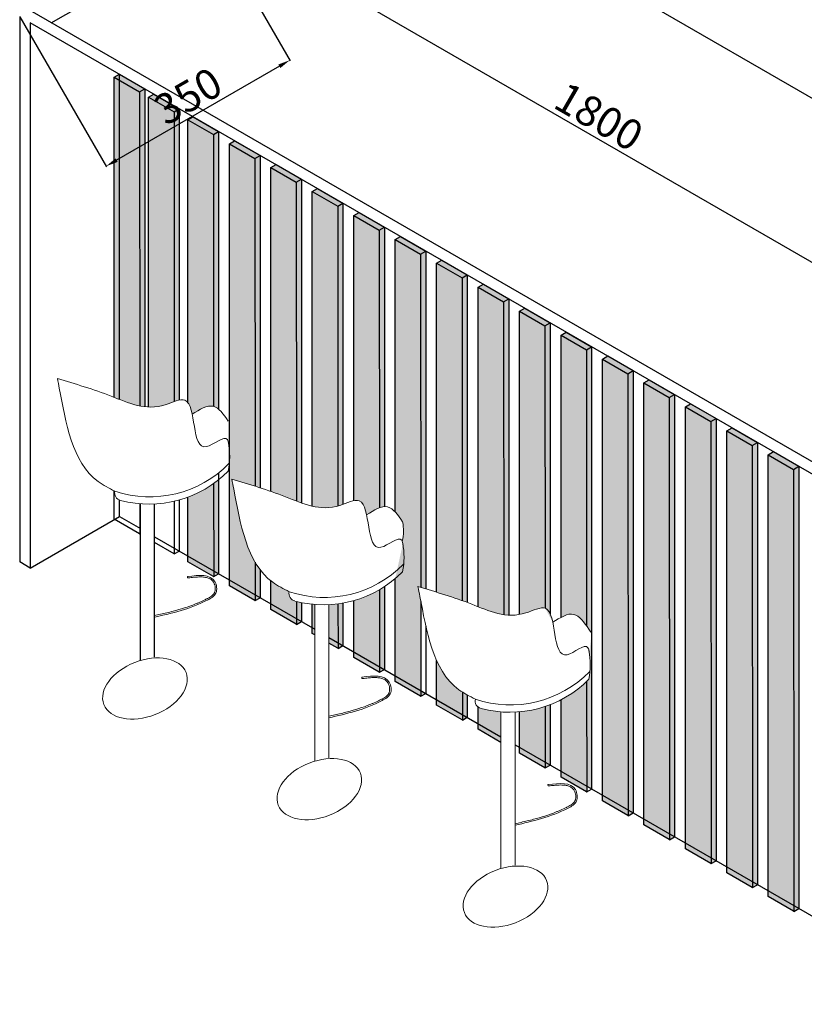
# Model space of a CAD drawing. Units: centimetres. Extents: x 209356 to 217348, y 253987 to 259034.
# Tile 1 of 7: x 209674 to 210968, y 254147 to 255772. Entities that reach past the tile are written whole.
import ezdxf

# ---------------------------------------------------------------- set-up
doc = ezdxf.new("R2010")
doc.units = ezdxf.units.CM
for name, color, linetype, lineweight in [('A-ANNO-DIMS', 2, 'Continuous', 18), ('A-ELEV', 7, 'Continuous', 25), ('A-ELEV-PATT', 32, 'Continuous', 13), ('A-FURN', 8, 'Continuous', 18)]:
    doc.layers.add(name, color=color, linetype=linetype, lineweight=lineweight)
doc.styles.get("Standard").update_dxf_attribs({"font": 'arial.ttf'})
doc.dimstyles.new('ISO-25', dxfattribs={"dimtxt": 50, "dimasz": 20, "dimexe": 1.25, "dimexo": 0.625, "dimtad": 1, "dimdec": 1, "dimtxsty": 'Standard', "dimcen": 2.5, "dimadec": 0, "dimazin": 0, "dimtfac": 1, "dimtdec": 1, "dimtmove": 0, "dimatfit": 3, "dimfxl": 1, "dimarcsym": 0})

# ---------------------------------------------------------------- blocks, each defined once
blk = doc.blocks.new('WOOD CHAIR')
for p, q in [((209213.3, 254105.5), (209213.3, 254643.6)), ((209261.5, 254116.4), (209261.5, 254642.8))]:
    blk.add_line(p, q)
for centre, radius, start, end in [((209261.7, 254806), 258.1, 348.8064, 10.7702), ((209245.8, 255048.2), 380.5, 251.5317, 315.539), ((209244, 255022.5), 380.1, 254.9145, 315.4643), ((209150.6, 254681), 26.1, 166.1036, 257.5958), ((209377.2, 254391.6), 2.77, 121.9926, 251.3474)]:
    blk.add_arc(centre, radius, start, end)
blk.add_ellipse((209228.8, 254009), major_axis=(141.2, 54.9), ratio=0.635047)
for points, knots in [([(209125.3, 254687.3), (209105.6, 254697.3), (208981, 254760.6), (208955.4, 254939), (208930.3, 255063), (208928.1, 255074)], [0, 0, 0, 0, 65.309963, 412.887053, 447.003391, 447.003391, 447.003391, 447.003391]), ([(208928.1, 255074), (208989.8, 255055.8), (209111.4, 255019.8), (209252.6, 254951.6), (209416.2, 255043.3), (209376.8, 254762.6), (209509.8, 254888.5), (209515.5, 254853.7), (209516.6, 254847.1)], [0, 0, 0, 0, 194.243648, 382.765289, 451.97711, 627.912461, 703.167603, 720.786202, 720.786202, 720.786202, 720.786202]), ([(209391.1, 254951.4), (209416.7, 254967.6), (209466.1, 254998.8), (209498.9, 254951.1), (209514.8, 254928)], [0, 0, 0, 0, 77.238961, 149.434731, 149.434731, 149.434731, 149.434731]), ([(209261.5, 254254.3), (209322.4, 254268), (209395, 254284.4), (209480, 254333), (209469.6, 254404.9), (209414.5, 254398.5), (209375.7, 254393.9)], [0, 0, 0, 0, 191.8386, 228.622109, 268.524723, 363.218072, 363.218072, 363.218072, 363.218072]), ([(209261.5, 254259.4), (209268.3, 254260.9), (209275.2, 254262.5), (209296.5, 254267.4), (209311, 254270.8), (209351.3, 254281.4), (209377.1, 254289.4), (209406.1, 254301.1), (209409.4, 254302.4), (209419.3, 254306.7), (209425.9, 254309.7), (209434.3, 254313.8), (209436.1, 254314.7), (209439.3, 254316.3), (209440.7, 254317), (209443.4, 254318.4), (209444.8, 254319.1), (209448.8, 254321.3), (209451.4, 254322.8), (209456.2, 254325.9), (209458.4, 254327.5), (209462.3, 254331), (209464, 254332.8), (209466.2, 254335.7), (209466.8, 254336.8), (209467.7, 254338.5), (209468, 254339.2), (209468.6, 254340.6), (209468.8, 254341.4), (209469.5, 254343.7), (209469.8, 254345.3), (209470.4, 254349.8), (209470.4, 254352.9), (209469.8, 254359), (209469.2, 254362), (209467.4, 254367.9), (209466.3, 254370.6), (209463.9, 254375), (209462.7, 254376.7), (209460.1, 254379.9), (209458.7, 254381.2), (209455.6, 254383.8), (209454, 254384.9), (209450.4, 254386.8), (209448.5, 254387.7), (209442.5, 254389.9), (209438.1, 254390.9), (209428.4, 254392.2), (209423.3, 254392.4), (209412.3, 254392.4), (209406.6, 254392), (209394.8, 254391.1), (209388.8, 254390.4), (209380.6, 254389.5), (209378.4, 254389.2), (209376.3, 254389)], [1.156813, 1.156813, 1.156813, 1.156813, 22.810617, 22.810617, 68.431852, 68.431852, 150.393922, 150.393922, 160.904538, 160.904538, 181.925769, 181.925769, 187.749873, 187.749873, 192.127257, 192.127257, 196.504641, 196.504641, 205.259408, 205.259408, 214.014175, 214.014175, 222.768943, 222.768943, 227.399514, 227.399514, 230.222361, 230.222361, 233.045208, 233.045208, 238.690903, 238.690903, 248.267073, 248.267073, 257.843243, 257.843243, 267.419412, 267.419412, 275.074878, 275.074878, 282.730344, 282.730344, 290.38581, 290.38581, 298.041276, 298.041276, 313.03296, 313.03296, 328.024645, 328.024645, 343.016329, 343.016329, 358.008014, 358.008014, 363.218072, 363.218072, 363.218072, 363.218072])]:
    blk.add_open_spline(points, degree=3, knots=knots)
blk = doc.blocks.new('FLUTED-PANEL')
for p, q in [((0, 753.9), (8.7, 758.9)), ((0, 24.5), (0, 753.9)), ((0, 753.9), (41.9, 729.7)), ((8.7, 758.9), (50.6, 734.7)), ((41.9, 729.7), (50.6, 734.7)), ((50.6, 734.7), (50.6, 4.7)), ((41.9, 729.7), (42.4, 0)), ((41.9, 0.3), (0, 24.5)), ((41.9, 0.3), (42.4, 0)), ((42.4, 0), (50.6, 4.7))]:
    blk.add_line(p, q)
blk = doc.blocks.new('*D12')
at = {"layer": 'A-ANNO-DIMS', "color": 0, "lineweight": -2, "transparency": 16777216}
for p, q in [((209691.8, 255787.1), (209834.6, 256034.4)), ((209851.3, 256023.4), (211375.5, 255143.4)), ((211250.7, 254887.1), (211393.5, 255134.4))]:
    blk.add_line(p, q, dxfattribs=at)
at = {"layer": 'A-ANNO-DIMS', "color": 0, "transparency": 16777216}
for points in [[(209853, 256026.3), (209849.6, 256020.5), (209834, 256033.4)], [(211377.2, 255146.3), (211373.9, 255140.5), (211392.8, 255133.4)]]:
    blk.add_solid(points, dxfattribs=at)
at = {"layer": 'Defpoints', "color": 0, "transparency": 16777216}
for p in [(209691.5, 255786.5), (211392.8, 255133.4), (211250.3, 254886.5)]:
    blk.add_point(p, dxfattribs=at)
at = {"layer": 'A-ANNO-DIMS', "color": 0, "transparency": 16777216, "insert": (210626.5, 255606), "char_height": 50, "attachment_point": 5, "rotation": 330}
blk.add_mtext('1800', dxfattribs=at)
blk = doc.blocks.new('*D34')
at = {"layer": 'A-ANNO-DIMS', "color": 0, "lineweight": -2, "transparency": 16777216}
for p, q in [((209977.6, 255951), (210120.4, 255703.6)), ((209674.5, 255776), (209817.3, 255528.6)), ((210102.5, 255694.7), (209834, 255539.7))]:
    blk.add_line(p, q, dxfattribs=at)
at = {"layer": 'A-ANNO-DIMS', "color": 0, "transparency": 16777216}
for points in [[(210100.8, 255697.6), (210104.1, 255691.8), (210119.8, 255704.7)], [(209832.3, 255542.6), (209835.7, 255536.8), (209816.7, 255529.7)]]:
    blk.add_solid(points, dxfattribs=at)
at = {"layer": 'Defpoints', "color": 0, "transparency": 16777216}
for p in [(209977.3, 255951.5), (209674.2, 255776.5), (209816.7, 255529.7)]:
    blk.add_point(p, dxfattribs=at)
at = {"layer": 'A-ANNO-DIMS', "color": 0, "transparency": 16777216, "insert": (209955.1, 255639.9), "char_height": 50, "attachment_point": 5, "rotation": 30}
blk.add_mtext('350', dxfattribs=at)

msp = doc.modelspace()

# ---------------------------------------------------------------- hatches: boundary and pattern name
at = {"layer": 'A-ELEV-PATT'}
h = msp.add_hatch(color=256, dxfattribs=at)
h.dxf.hatch_style = 1
h.paths.add_polyline_path([(209838.7169, 255681.5492), (209830.0636, 255676.5532), (209871.9793, 255652.3531), (209880.6326, 255657.3491)])
h.paths.add_polyline_path([(209872.3394, 255134.0549), (209880.6326, 255132.7439), (209880.6326, 255657.3491), (209871.9793, 255652.3531)])
h.paths.add_polyline_path([(209871.6996, 255134.2031), (209872.3394, 255134.0785), (209871.9793, 255652.3531), (209830.0636, 255676.5532), (209830.0636, 255148.2775), (209832.6333, 255147.2538), (209835.2039, 255146.2291), (209837.7762, 255145.2078), (209840.3508, 255144.1942), (209842.9285, 255143.1925), (209845.5101, 255142.2073), (209848.0963, 255141.2426), (209850.6877, 255140.3029), (209853.2852, 255139.3926), (209855.8896, 255138.5158), (209858.5014, 255137.677), (209861.1216, 255136.8804), (209863.7507, 255136.1304), (209866.3896, 255135.4313), (209869.039, 255134.7874)])
h = msp.add_hatch(color=256, dxfattribs=at)
h.dxf.hatch_style = 1
h.paths.add_polyline_path([(209895.4569, 255648.7903), (209886.8036, 255643.7943), (209928.7193, 255619.5942), (209937.3726, 255624.5902)])
h.paths.add_polyline_path([(209886.8036, 255132.2353), (209889.7902, 255132.1482), (209892.7967, 255132.1701), (209895.8239, 255132.3066), (209898.873, 255132.5631), (209901.9447, 255132.9452), (209905.0401, 255133.4584), (209908.16, 255134.1083), (209911.3054, 255134.9002), (209914.4774, 255135.8398), (209917.6725, 255136.9213), (209920.8723, 255138.0978), (209924.0546, 255139.3129), (209927.1973, 255140.5103), (209929.0517, 255141.1863), (209928.7193, 255619.5942), (209886.8036, 255643.7943)])
h = msp.add_hatch(color=256, dxfattribs=at)
h.dxf.hatch_style = 1
edge = h.paths.add_edge_path()
edge.add_line((209937.3726, 255624.5902), (209928.7193, 255619.5942))
edge.add_line((209928.7193, 255619.5942), (209929.0517, 255141.1956))
edge.add_spline(control_points=[(209929.0517, 255141.1956), (209931.9533, 255142.248), (209934.7548, 255143.1561), (209937.3726, 255143.7067)], knot_values=[411.187631291, 411.187631291, 411.187631291, 411.187631291, 428.578941434, 428.578941434, 428.578941434, 428.578941434], degree=3, periodic=0)
edge.add_line((209937.3726, 255143.7067), (209937.3726, 255624.5902))
edge = h.paths.add_edge_path()
edge.add_line((209993.6447, 255582.1096), (209951.7289, 255606.3096))
edge.add_line((209951.7289, 255606.3096), (209951.7289, 255139.4147))
edge.add_spline(control_points=[(209951.7289, 255139.4147), (209954.9954, 255135.0962), (209957.0859, 255128.2201), (209958.7321, 255120.3781)], knot_values=[468.970685224, 468.970685224, 468.970685224, 468.970685224, 508.024917649, 508.024917649, 508.024917649, 508.024917649], degree=3, periodic=0)
edge.add_spline(control_points=[(209958.7321, 255120.3781), (209971.0125, 255128.1269), (209983.5055, 255136.01), (209993.7821, 255133.4155), (209993.9564, 255133.3684)], knot_values=[0, 0, 0, 0, 77.238961281, 78.57658104, 78.57658104, 78.57658104, 78.57658104], degree=3, periodic=0)
edge.add_line((209993.9564, 255133.3684), (209993.6447, 255582.1096))
h = msp.add_hatch(color=256, dxfattribs=at)
h.dxf.hatch_style = 1
h.paths.add_polyline_path([(209960.3823, 255611.3056), (209951.7289, 255606.3096), (209993.6447, 255582.1096), (210002.298, 255587.1056)])
edge = h.paths.add_edge_path()
edge.add_arc((209888.0616, 255154.5395), 182.5816, 290.4081991, 305.4836992)
edge.add_line((209994.045, 255005.8668), (209994.1516, 254852.4022))
edge.add_line((209994.1516, 254852.4022), (209951.7289, 254876.895))
edge.add_line((209951.7289, 254876.895), (209951.7289, 254983.4181))
edge = h.paths.add_edge_path()
edge.add_arc((209888.0616, 255154.5395), 182.5816, 305.4836992, 308.7315997)
edge.add_line((210002.298, 255012.1102), (210002.298, 254857.1056))
edge.add_line((210002.298, 254857.1056), (209994.1516, 254852.4022))
edge.add_line((209994.1516, 254852.4022), (209994.045, 255005.8668))
h.paths.add_polyline_path([(209993.9565, 255133.3142), (209994.8652, 255133.094), (209997.4235, 255132.0135), (209999.8981, 255130.5369), (210002.298, 255128.7074), (210002.298, 255587.1056), (209993.6447, 255582.1096)])
h.paths.add_polyline_path([(210001.5192, 255076.2748), (210001.1006, 255076.0389), (210002.1063, 255076.5853)])
h.paths.add_polyline_path([(209996.6216, 255073.4867), (209994.8818, 255072.491), (209995.4223, 255072.7972)])
h.paths.add_polyline_path([(209994.0875, 255072.0409), (209993.9991, 255071.9919), (209993.9991, 255071.9908)])
h.paths.add_polyline_path([(209999.286, 255075.0167), (209999.2266, 255074.9826), (209999.4643, 255075.1166)])
h.paths.add_polyline_path([(209993.9991, 255071.9857), (209994.3441, 255072.1832), (209993.9991, 255071.9919)])
h = msp.add_hatch(color=256, dxfattribs=at)
h.dxf.hatch_style = 1
edge = h.paths.add_edge_path()
edge.add_line((210062.018, 255542.6342), (210020.1023, 255566.8343))
edge.add_line((210020.1023, 255566.8343), (210020.1023, 255061.2706))
edge.add_arc((209896.5952, 255050.551), 123.9714, -4.9604263, 4.9604263, ccw=False)
edge.add_line((210020.1023, 255039.8315), (210020.1023, 254846.8263))
edge.add_line((210020.1023, 254846.8263), (210062.5184, 254822.3373))
edge.add_line((210062.5184, 254822.3373), (210062.481, 254876.2165))
edge.add_spline(control_points=[(210062.481, 254876.2165), (210042.2873, 254910.7685), (210034.11, 254963.1736), (210025.0707, 255007.8633), (210023.9948, 255013.1827)], knot_values=[160.382869641, 160.382869641, 160.382869641, 160.382869641, 412.887053283, 447.00339111, 447.00339111, 447.00339111, 447.00339111], degree=3, periodic=0)
edge.add_spline(control_points=[(210023.9948, 255013.1827), (210036.8013, 255009.3967), (210049.6079, 255005.6107), (210062.3939, 255001.6068)], knot_values=[0, 0, 0, 0, 83.916340246, 83.916340246, 83.916340246, 83.916340246], degree=3, periodic=0)
edge.add_line((210062.3939, 255001.6068), (210062.018, 255542.6342))
edge = h.paths.add_edge_path()
edge.add_line((210070.6713, 255547.6302), (210062.018, 255542.6342))
edge.add_line((210062.018, 255542.6342), (210062.3939, 255001.6068))
edge.add_spline(control_points=[(210062.3939, 255001.6068), (210065.154, 255000.7425), (210067.9133, 254999.868), (210070.6713, 254998.9811)], knot_values=[83.916340246, 83.916340246, 83.916340246, 83.916340246, 102.031847918, 102.031847918, 102.031847918, 102.031847918], degree=3, periodic=0)
edge.add_line((210070.6713, 254998.9811), (210070.6713, 255547.6302))
h = msp.add_hatch(color=256, dxfattribs=at)
h.dxf.hatch_style = 1
h.paths.add_polyline_path([(210028.7556, 255571.8303), (210020.1023, 255566.8343), (210062.018, 255542.6342), (210070.6713, 255547.6302)])
h.paths.add_polyline_path([(210062.5184, 254822.3373), (210020.1023, 254846.8263), (210020.1023, 254837.4196), (210062.5249, 254812.9269)])
h.paths.add_polyline_path([(210070.6713, 254817.6302), (210062.5184, 254822.3373), (210062.5249, 254812.9269)])
h = msp.add_hatch(color=256, dxfattribs=at)
h.dxf.hatch_style = 1
h.paths.add_polyline_path([(210097.1289, 255532.3549), (210088.4756, 255527.3589), (210130.3913, 255503.1589), (210139.0446, 255508.1548)])
h = msp.add_hatch(color=256, dxfattribs=at)
h.dxf.hatch_style = 1
edge = h.paths.add_edge_path()
edge.add_line((210130.3913, 255503.1589), (210088.4756, 255527.3589))
edge.add_line((210088.4756, 255527.3589), (210088.4756, 254993.0564))
edge.add_spline(control_points=[(210088.4756, 254993.0564), (210096.5563, 254990.2663), (210110.6625, 254985.1298), (210124.7103, 254979.3735), (210130.7568, 254977.0458)], knot_values=[141.052694506, 141.052694506, 141.052694506, 141.052694506, 194.243647816, 234.067349628, 234.067349628, 234.067349628, 234.067349628], degree=3, periodic=0)
edge.add_line((210130.7568, 254977.0458), (210130.3913, 255503.1589))
edge = h.paths.add_edge_path()
edge.add_line((210198.7647, 255463.6835), (210156.8489, 255487.8836))
edge.add_line((210156.8489, 255487.8836), (210156.8489, 254968.6697))
edge.add_spline(control_points=[(210156.8489, 254968.6697), (210170.3528, 254965.5595), (210184.2937, 254964.768), (210199.1084, 254968.8528)], knot_values=[290.654547314, 290.654547314, 290.654547314, 290.654547314, 377.058614809, 377.058614809, 377.058614809, 377.058614809], degree=3, periodic=0)
edge.add_line((210199.1084, 254968.8528), (210198.7647, 255463.6835))
edge = h.paths.add_edge_path()
edge.add_line((210267.138, 255424.2081), (210225.2222, 255448.4082))
edge.add_line((210225.2222, 255448.4082), (210225.2222, 254977.6598))
edge.add_spline(control_points=[(210225.2222, 254977.6598), (210228.6719, 254978.3656), (210239.4144, 254978.6135), (210244.0368, 254965.5476), (210246.3993, 254954.2934)], knot_values=[428.983516451, 428.983516451, 428.983516451, 428.983516451, 451.977109906, 508.024917649, 508.024917649, 508.024917649, 508.024917649], degree=3, periodic=0)
edge.add_spline(control_points=[(210246.3993, 254954.2934), (210253.5599, 254958.8116), (210260.7204, 254963.3299), (210267.4564, 254965.8411)], knot_values=[0, 0, 0, 0, 45.037191144, 45.037191144, 45.037191144, 45.037191144], degree=3, periodic=0)
edge.add_line((210267.4564, 254965.8411), (210267.138, 255424.2081))
h = msp.add_hatch(color=256, dxfattribs=at)
h.dxf.hatch_style = 1
edge = h.paths.add_edge_path()
edge.add_line((210139.0446, 255508.1548), (210130.3913, 255503.1589))
edge.add_line((210130.3913, 255503.1589), (210130.7568, 254977.0458))
edge.add_spline(control_points=[(210130.7568, 254977.0458), (210133.5114, 254975.9853), (210136.2727, 254974.9532), (210139.0446, 254973.9732)], knot_values=[234.067349628, 234.067349628, 234.067349628, 234.067349628, 252.209805879, 252.209805879, 252.209805879, 252.209805879], degree=3, periodic=0)
edge.add_line((210139.0446, 254973.9732), (210139.0446, 255508.1548))
edge = h.paths.add_edge_path()
edge.add_line((210207.418, 255468.6795), (210198.7647, 255463.6835))
edge.add_line((210198.7647, 255463.6835), (210199.1084, 254968.8528))
edge.add_spline(control_points=[(210199.1084, 254968.8528), (210200.0869, 254969.1225), (210202.8425, 254969.939), (210205.6292, 254970.9288), (210207.418, 254971.5931)], knot_values=[377.058614809, 377.058614809, 377.058614809, 377.058614809, 382.765289469, 393.068098738, 393.068098738, 393.068098738, 393.068098738], degree=3, periodic=0)
edge.add_line((210207.418, 254971.5931), (210207.418, 255468.6795))
edge = h.paths.add_edge_path()
edge.add_line((210275.7913, 255429.2041), (210267.138, 255424.2081))
edge.add_line((210267.138, 255424.2081), (210267.4564, 254965.8411))
edge.add_spline(control_points=[(210267.4564, 254965.8411), (210270.3225, 254966.9096), (210273.1117, 254967.6148), (210275.7913, 254967.802)], knot_values=[45.037191144, 45.037191144, 45.037191144, 45.037191144, 64.199838197, 64.199838197, 64.199838197, 64.199838197], degree=3, periodic=0)
edge.add_line((210275.7913, 254967.802), (210275.7913, 255429.2041))
h = msp.add_hatch(color=256, dxfattribs=at)
h.dxf.hatch_style = 1
h.paths.add_polyline_path([(210165.5022, 255492.8796), (210156.8489, 255487.8836), (210198.7647, 255463.6835), (210207.418, 255468.6795)])
h = msp.add_hatch(color=256, dxfattribs=at)
h.dxf.hatch_style = 1
h.paths.add_polyline_path([(210233.8755, 255453.4042), (210225.2222, 255448.4082), (210267.138, 255424.2081), (210275.7913, 255429.2041)])
edge = h.paths.add_edge_path()
edge.add_arc((210175.7288, 254988.4547), 182.5816, 300.1924839, 303.2328114)
edge.add_line((210275.7913, 254835.7342), (210275.7913, 254699.2041))
edge.add_line((210275.7913, 254699.2041), (210267.6449, 254694.5008))
edge.add_line((210267.6449, 254694.5008), (210267.5503, 254830.642))
edge = h.paths.add_edge_path()
edge.add_arc((210175.7288, 254988.4547), 182.5816, 285.7282758, 300.1924839)
edge.add_line((210267.5503, 254830.642), (210267.6449, 254694.5008))
edge.add_line((210267.6449, 254694.5008), (210225.2222, 254718.9936))
edge.add_line((210225.2222, 254718.9936), (210225.2222, 254812.7093))
h = msp.add_hatch(color=256, dxfattribs=at)
h.dxf.hatch_style = 1
edge = h.paths.add_edge_path()
edge.add_line((210335.5113, 255384.7328), (210293.5956, 255408.9329))
edge.add_line((210293.5956, 255408.9329), (210293.5956, 254959.1517))
edge.add_spline(control_points=[(210293.5956, 254959.1517), (210297.8374, 254954.6317), (210301.8122, 254948.8491), (210305.787, 254943.0666)], knot_values=[111.704744255, 111.704744255, 111.704744255, 111.704744255, 149.434731389, 149.434731389, 149.434731389, 149.434731389], degree=3, periodic=0)
edge.add_arc((210232.7205, 254928.0817), 74.5872, -13.5167625, 11.5898438, ccw=False)
edge.add_spline(control_points=[(210305.2418, 254910.6484), (210305.8981, 254908.8541), (210306.2766, 254906.5205), (210306.6552, 254904.1869)], knot_values=[707.821270708, 707.821270708, 707.821270708, 707.821270708, 720.786201866, 720.786201866, 720.786201866, 720.786201866], degree=3, periodic=0)
edge.add_arc((210184.2624, 254884.4663), 123.9714, 9.9291308, 11.134566, ccw=False)
edge.add_spline(control_points=[(210306.6552, 254904.1869), (210306.2766, 254906.5205), (210305.8981, 254908.8541), (210305.2418, 254910.6484)], knot_values=[707.821270708, 707.821270708, 707.821270708, 707.821270708, 720.786201866, 720.786201866, 720.786201866, 720.786201866], degree=3, periodic=0)
edge.add_arc((210184.2624, 254884.4663), 123.9714, -11.1935567, 10.3654744, ccw=False)
edge.add_arc((210175.7288, 254988.4547), 182.5816, 310.2074031, 315.4643031, ccw=False)
edge.add_line((210293.5956, 254849.0148), (210293.5956, 254688.9248))
edge.add_line((210293.5956, 254688.9248), (210336.0117, 254664.4359))
edge.add_line((210336.0117, 254664.4359), (210335.9095, 254811.4969))
edge.add_spline(control_points=[(210335.9095, 254811.4969), (210335.3731, 254814.2946), (210333.7804, 254822.5539), (210332.1599, 254830.5652), (210331.084, 254835.8846)], knot_values=[395.621930027, 395.621930027, 395.621930027, 395.621930027, 412.887053283, 447.00339111, 447.00339111, 447.00339111, 447.00339111], degree=3, periodic=0)
edge.add_spline(control_points=[(210331.084, 254835.8846), (210332.6872, 254835.4107), (210334.2904, 254834.9367), (210335.8936, 254834.4624)], knot_values=[0, 0, 0, 0, 10.505199123, 10.505199123, 10.505199123, 10.505199123], degree=3, periodic=0)
edge.add_line((210335.8936, 254834.4624), (210335.5113, 255384.7328))
h = msp.add_hatch(color=256, dxfattribs=at)
h.dxf.hatch_style = 1
h.paths.add_polyline_path([(210302.2489, 255413.9288), (210293.5956, 255408.9329), (210335.5113, 255384.7328), (210344.1646, 255389.7288)])
h.paths.add_polyline_path([(210336.0117, 254664.4359), (210293.5956, 254688.9248), (210293.5956, 254679.5182), (210336.0182, 254655.0255)])
h.paths.add_polyline_path([(210344.1646, 254659.7288), (210336.0117, 254664.4359), (210336.0182, 254655.0255)])
h = msp.add_hatch(color=256, dxfattribs=at)
h.dxf.hatch_style = 1
edge = h.paths.add_edge_path()
edge.add_line((210344.1646, 255389.7288), (210335.5113, 255384.7328))
edge.add_line((210335.5113, 255384.7328), (210335.8936, 254834.4624))
edge.add_spline(control_points=[(210335.8936, 254834.4624), (210338.6508, 254833.6465), (210341.4079, 254832.8294), (210344.1646, 254832.0088)], knot_values=[10.505199123, 10.505199123, 10.505199123, 10.505199123, 28.572517978, 28.572517978, 28.572517978, 28.572517978], degree=3, periodic=0)
edge.add_line((210344.1646, 254832.0088), (210344.1646, 255389.7288))
h = msp.add_hatch(color=256, dxfattribs=at)
h.dxf.hatch_style = 1
h.paths.add_polyline_path([(210370.6222, 255374.4535), (210361.9689, 255369.4575), (210403.8846, 255345.2574), (210412.5379, 255350.2534)])
h.paths.add_polyline_path([(210412.5379, 254620.2534), (210404.385, 254624.9605), (210404.3915, 254615.5501)])
h.paths.add_polyline_path([(210404.385, 254624.9605), (210361.9689, 254649.4495), (210361.9689, 254640.0428), (210404.3915, 254615.5501)])
h = msp.add_hatch(color=256, dxfattribs=at)
h.dxf.hatch_style = 1
edge = h.paths.add_edge_path()
edge.add_line((210403.8846, 255345.2574), (210361.9689, 255369.4575))
edge.add_line((210361.9689, 255369.4575), (210361.9689, 254826.6377))
edge.add_spline(control_points=[(210361.9689, 254826.6377), (210376.0935, 254822.3021), (210390.198, 254817.7529), (210404.2546, 254812.6966)], knot_values=[67.482286261, 67.482286261, 67.482286261, 67.482286261, 160.131888062, 160.131888062, 160.131888062, 160.131888062], degree=3, periodic=0)
edge.add_line((210404.2546, 254812.6966), (210403.8846, 255345.2574))
h = msp.add_hatch(color=256, dxfattribs=at)
h.dxf.hatch_style = 1
edge = h.paths.add_edge_path()
edge.add_line((210412.5379, 255350.2534), (210403.8846, 255345.2574))
edge.add_line((210403.8846, 255345.2574), (210404.2546, 254812.6966))
edge.add_spline(control_points=[(210404.2546, 254812.6966), (210407.0176, 254811.7027), (210409.7788, 254810.6893), (210412.5379, 254809.654)], knot_values=[160.131888062, 160.131888062, 160.131888062, 160.131888062, 178.343545798, 178.343545798, 178.343545798, 178.343545798], degree=3, periodic=0)
edge.add_line((210412.5379, 254809.654), (210412.5379, 255350.2534))
h = msp.add_hatch(color=256, dxfattribs=at)
h.dxf.hatch_style = 1
h.paths.add_polyline_path([(210438.9955, 255334.9781), (210430.3422, 255329.9821), (210472.2579, 255305.7821), (210480.9113, 255310.7781)])
h = msp.add_hatch(color=256, dxfattribs=at)
h.dxf.hatch_style = 1
edge = h.paths.add_edge_path()
edge.add_line((210472.2579, 255305.7821), (210430.3422, 255329.9821))
edge.add_line((210430.3422, 255329.9821), (210430.3422, 254802.6944))
edge.add_spline(control_points=[(210430.3422, 254802.6944), (210444.1853, 254797.1865), (210458.104, 254791.8527), (210472.6164, 254789.7267)], knot_values=[217.563869727, 217.563869727, 217.563869727, 217.563869727, 309.028485894, 309.028485894, 309.028485894, 309.028485894], degree=3, periodic=0)
edge.add_line((210472.6164, 254789.7267), (210472.2579, 255305.7821))
h = msp.add_hatch(color=256, dxfattribs=at)
h.dxf.hatch_style = 1
edge = h.paths.add_edge_path()
edge.add_line((210480.9113, 255310.7781), (210472.2579, 255305.7821))
edge.add_line((210472.2579, 255305.7821), (210472.6164, 254789.7267))
edge.add_spline(control_points=[(210472.6164, 254789.7267), (210475.359, 254789.3249), (210478.1228, 254789.0377), (210480.9113, 254788.8855)], knot_values=[309.028485894, 309.028485894, 309.028485894, 309.028485894, 326.313488296, 326.313488296, 326.313488296, 326.313488296], degree=3, periodic=0)
edge.add_line((210480.9113, 254788.8855), (210480.9113, 255310.7781))
h = msp.add_hatch(color=256, dxfattribs=at)
h.dxf.hatch_style = 1
h.paths.add_polyline_path([(210507.3688, 255295.5028), (210498.7155, 255290.5068), (210540.6313, 255266.3067), (210549.2846, 255271.3027)])
edge = h.paths.add_edge_path()
edge.add_arc((210482.818, 254811.1567), 182.5816, 274.9951075, 288.6044838)
edge.add_line((210541.0677, 254638.1162), (210541.1382, 254536.5994))
edge.add_line((210541.1382, 254536.5994), (210498.7155, 254561.0921))
edge.add_line((210498.7155, 254561.0921), (210498.7155, 254629.2685))
edge = h.paths.add_edge_path()
edge.add_arc((210482.818, 254811.1567), 182.5816, 288.6044838, 291.3483603)
edge.add_line((210549.2846, 254641.1031), (210549.2846, 254541.3027))
edge.add_line((210549.2846, 254541.3027), (210541.1382, 254536.5994))
edge.add_line((210541.1382, 254536.5994), (210541.0677, 254638.1162))
h = msp.add_hatch(color=256, dxfattribs=at)
h.dxf.hatch_style = 1
edge = h.paths.add_edge_path()
edge.add_line((210540.6313, 255266.3067), (210498.7155, 255290.5068))
edge.add_line((210498.7155, 255290.5068), (210498.7155, 254789.8817))
edge.add_spline(control_points=[(210498.7155, 254789.8817), (210502.1454, 254790.472), (210517.4101, 254794.1527), (210543.8007, 254808.9556), (210551.126, 254788.2496), (210553.4885, 254776.9953)], knot_values=[362.369570317, 362.369570317, 362.369570317, 362.369570317, 382.765289469, 451.977109906, 508.024917649, 508.024917649, 508.024917649, 508.024917649], degree=3, periodic=0)
edge.add_line((210540.955, 254800.2404), (210540.6313, 255266.3067))
edge = h.paths.add_edge_path(flags=17)
edge.add_line((210549.2846, 255271.3027), (210540.6313, 255266.3067))
edge.add_line((210540.6313, 255266.3067), (210540.955, 254800.2846))
edge.add_spline(control_points=[(210540.955, 254800.2846), (210541.1368, 254800.2232), (210544.7056, 254798.9022), (210547.3296, 254795.5258), (210549.2846, 254791.151)], knot_values=[450.415519807, 450.415519807, 450.415519807, 450.415519807, 451.977109906, 481.471652475, 481.471652475, 481.471652475, 481.471652475], degree=3, periodic=0)
edge.add_line((210549.2846, 254791.151), (210549.2846, 255271.3027))
h = msp.add_hatch(color=256, dxfattribs=at)
h.dxf.hatch_style = 1
h.paths.add_polyline_path([(210575.7422, 255256.0274), (210567.0888, 255251.0314), (210609.0046, 255226.8314), (210617.6579, 255231.8274)])
h.paths.add_polyline_path([(210609.505, 254506.5344), (210567.0888, 254531.0234), (210567.0888, 254521.6168), (210609.5115, 254497.124)])
h = msp.add_hatch(color=256, dxfattribs=at)
h.dxf.hatch_style = 1
edge = h.paths.add_edge_path()
edge.add_line((210609.0046, 255226.8314), (210567.0888, 255251.0314))
edge.add_line((210567.0888, 255251.0314), (210567.0888, 254785.1249))
edge.add_spline(control_points=[(210567.0888, 254785.1249), (210574.6127, 254789.1096), (210590.8871, 254794.7518), (210602.86, 254780.0604), (210609.3213, 254770.8967)], knot_values=[28.745104313, 28.745104313, 28.745104313, 28.745104313, 77.238961281, 138.209017936, 138.209017936, 138.209017936, 138.209017936], degree=3, periodic=0)
edge.add_line((210609.3213, 254770.8967), (210609.0046, 255226.8314))
edge = h.paths.add_edge_path()
edge.add_line((210617.6579, 255231.8274), (210609.0046, 255226.8314))
edge.add_line((210609.0046, 255226.8314), (210609.3213, 254770.8967))
edge.add_spline(control_points=[(210609.3213, 254770.8967), (210610.511, 254769.2095), (210611.6936, 254767.489), (210612.8762, 254765.7686)], knot_values=[138.209017936, 138.209017936, 138.209017936, 138.209017936, 149.434731389, 149.434731389, 149.434731389, 149.434731389], degree=3, periodic=0)
edge.add_arc((210567.5561, 254726.927), 59.6873, 32.9227648, 40.5982268, ccw=False)
edge.add_line((210617.6579, 254759.3675), (210617.6579, 255231.8274))
h = msp.add_hatch(color=256, dxfattribs=at)
h.dxf.hatch_style = 1
h.paths.add_polyline_path([(210644.1155, 255216.5521), (210635.4622, 255211.5561), (210677.3779, 255187.356), (210686.0312, 255192.352)])
h.paths.add_polyline_path([(210677.8848, 254457.6487), (210686.0312, 254462.352), (210686.0312, 255192.352), (210677.3779, 255187.356)])
h.paths.add_polyline_path([(210635.4622, 254482.1414), (210677.8848, 254457.6487), (210677.3779, 255187.356), (210635.4622, 255211.5561)])
h = msp.add_hatch(color=256, dxfattribs=at)
h.dxf.hatch_style = 1
h.paths.add_polyline_path([(210712.4888, 255177.0767), (210703.8355, 255172.0807), (210745.7512, 255147.8807), (210754.4045, 255152.8766)])
h.paths.add_polyline_path([(210746.2582, 254418.1733), (210754.4045, 254422.8766), (210754.4045, 255152.8766), (210745.7512, 255147.8807)])
h.paths.add_polyline_path([(210703.8355, 254442.6661), (210746.2582, 254418.1733), (210745.7512, 255147.8807), (210703.8355, 255172.0807)])
h = msp.add_hatch(color=256, dxfattribs=at)
h.dxf.hatch_style = 1
h.paths.add_polyline_path([(210780.8621, 255137.6014), (210772.2088, 255132.6054), (210814.1246, 255108.4053), (210822.7779, 255113.4013)])
h.paths.add_polyline_path([(210814.6315, 254378.698), (210822.7779, 254383.4013), (210822.7779, 255113.4013), (210814.1246, 255108.4053)])
h.paths.add_polyline_path([(210772.2088, 254403.1907), (210814.6315, 254378.698), (210814.1246, 255108.4053), (210772.2088, 255132.6054)])
h = msp.add_hatch(color=256, dxfattribs=at)
h.dxf.hatch_style = 1
h.paths.add_polyline_path([(210849.2354, 255098.126), (210840.5821, 255093.13), (210882.4979, 255068.9299), (210891.1512, 255073.9259)])
h.paths.add_polyline_path([(210883.0048, 254339.2226), (210891.1512, 254343.9259), (210891.1512, 255073.9259), (210882.4979, 255068.9299)])
h.paths.add_polyline_path([(210840.5821, 254363.7154), (210883.0048, 254339.2226), (210882.4979, 255068.9299), (210840.5821, 255093.13)])
h = msp.add_hatch(color=256, dxfattribs=at)
h.dxf.hatch_style = 1
h.paths.add_polyline_path([(210917.6088, 255058.6506), (210908.9555, 255053.6546), (210950.8712, 255029.4546), (210959.5245, 255034.4506)])
h.paths.add_polyline_path([(210951.3781, 254299.7473), (210959.5245, 254304.4506), (210959.5245, 255034.4506), (210950.8712, 255029.4546)])
h.paths.add_polyline_path([(210908.9555, 254324.24), (210951.3781, 254299.7473), (210950.8712, 255029.4546), (210908.9555, 255053.6546)])
h = msp.add_hatch(color=256, dxfattribs=at)
h.dxf.hatch_style = 1
edge = h.paths.add_edge_path()
edge.add_spline(control_points=[(210070.6713, 254863.862), (210067.7214, 254867.7766), (210065.0001, 254871.9062), (210062.481, 254876.2165)], knot_values=[128.883300955, 128.883300955, 128.883300955, 128.883300955, 160.382869641, 160.382869641, 160.382869641, 160.382869641], degree=3, periodic=0)
edge.add_line((210062.481, 254876.2165), (210062.5184, 254822.3373))
edge.add_line((210062.5184, 254822.3373), (210070.6713, 254817.6302))
edge.add_line((210070.6713, 254817.6302), (210070.6713, 254863.862))
h.paths.add_polyline_path([(210088.4756, 254807.3509), (210088.4756, 254797.9443), (210130.3913, 254773.7442), (210130.8983, 254773.4515), (210130.8917, 254782.8619)])
edge = h.paths.add_edge_path()
edge.add_arc((210175.7288, 254988.4547), 182.5816, 254.9144881, 255.7778696, ccw=False)
edge.add_arc((210130.9033, 254824.4104), 12.5379, 166.1035689, 257.5957769, ccw=False)
edge.add_spline(control_points=[(210118.7324, 254827.4216), (210109.2654, 254832.2301), (210098.6031, 254837.6458), (210089.4795, 254844.6095), (210088.4756, 254845.4091)], knot_values=[0, 0, 0, 0, 65.309963166, 73.556041403, 73.556041403, 73.556041403, 73.556041403], degree=3, periodic=0)
edge.add_line((210088.4756, 254845.4091), (210088.4756, 254807.3509))
edge.add_line((210088.4756, 254807.3509), (210130.8917, 254782.8619))
edge.add_line((210130.8917, 254782.8619), (210130.8718, 254811.4691))
h.paths.add_polyline_path([(210139.0446, 254809.5964, -0.011482161), (210130.8718, 254811.4691), (210130.8917, 254782.8619), (210139.0446, 254778.1548)])
h.paths.add_polyline_path([(210130.8917, 254782.8619), (210130.8983, 254773.4515), (210139.0446, 254778.1548)])
h = msp.add_hatch(color=256, dxfattribs=at)
h.dxf.hatch_style = 1
h.paths.add_polyline_path([(210161.0165, 254806.4668, -0.005730997), (210156.8489, 254806.8519), (210156.8489, 254767.8755), (210161.0165, 254765.4694)])
h.paths.add_polyline_path([(210161.0165, 254765.4694), (210156.8489, 254767.8755), (210156.8489, 254758.4689), (210161.0165, 254756.0627)])
h.paths.add_polyline_path([(210199.2206, 254807.3907, -0.020749851), (210184.1309, 254806.0665), (210184.1309, 254752.1243), (210199.265, 254743.3866)])
h.paths.add_polyline_path([(210184.1309, 254752.1243), (210184.1309, 254742.7176), (210198.7647, 254734.2688), (210199.2716, 254733.9762), (210199.265, 254743.3866)])
h.paths.add_polyline_path([(210207.418, 254808.6441, -0.011356196), (210199.2206, 254807.3907), (210199.265, 254743.3866), (210207.418, 254738.6795)])
h.paths.add_polyline_path([(210199.265, 254743.3866), (210199.2716, 254733.9762), (210207.418, 254738.6795)])
h = msp.add_hatch(color=256, dxfattribs=at)
h.dxf.hatch_style = 1
h.paths.add_polyline_path([(210617.6579, 254759.3675), (210613.7444, 254726.8889, -0.089013219), (210612.9647, 254683.1024, -0.006893451), (210609.3848, 254679.563), (210609.505, 254506.5344), (210617.6579, 254501.8274)])
h = msp.add_hatch(color=256, dxfattribs=at)
h.dxf.hatch_style = 1
edge = h.paths.add_edge_path()
edge.add_spline(control_points=[(210404.3594, 254661.8817), (210402.3989, 254663.1254), (210383.5593, 254675.8421), (210370.6424, 254694.5177), (210361.9689, 254713.7236)], knot_values=[50.655423077, 50.655423077, 50.655423077, 50.655423077, 65.309963166, 194.96587381, 194.96587381, 194.96587381, 194.96587381], degree=3, periodic=0)
edge.add_line((210361.9689, 254713.7236), (210361.9689, 254649.4495))
edge.add_line((210361.9689, 254649.4495), (210404.385, 254624.9605))
edge.add_line((210404.385, 254624.9605), (210404.3594, 254661.8817))
edge = h.paths.add_edge_path()
edge.add_spline(control_points=[(210412.5379, 254657.0641), (210409.7477, 254658.6055), (210407.0102, 254660.2001), (210404.3594, 254661.8817)], knot_values=[30.84038343, 30.84038343, 30.84038343, 30.84038343, 50.655423077, 50.655423077, 50.655423077, 50.655423077], degree=3, periodic=0)
edge.add_line((210404.3594, 254661.8817), (210404.385, 254624.9605))
edge.add_line((210404.385, 254624.9605), (210412.5379, 254620.2534))
edge.add_line((210412.5379, 254620.2534), (210412.5379, 254657.0641))
h = msp.add_hatch(color=256, dxfattribs=at)
h.dxf.hatch_style = 1
h.paths.add_polyline_path([(210609.3848, 254679.563, -0.071668587), (210567.0888, 254649.1861), (210567.0888, 254531.0234), (210609.505, 254506.5344)])
h = msp.add_hatch(color=256, dxfattribs=at)
h.dxf.hatch_style = 1
h.paths.add_polyline_path([(210468.1057, 254629.1688, -0.045688015), (210435.2993, 254634.8671, -0.110391257), (210430.3422, 254637.179), (210430.3422, 254609.9741), (210468.1057, 254588.1713)])
h.paths.add_polyline_path([(210430.3422, 254609.9741), (210430.3422, 254600.5675), (210468.1057, 254578.7647), (210468.1057, 254588.1713)])

# ---------------------------------------------------------------- linework, layer by layer
at = {"layer": 'A-ELEV'}
for p, q in [((211769.9535, 255186.5492), (210211.1078, 256086.5492)), ((209726.1336, 255766.5492), (210245.7488, 256066.5492)), ((209674.1721, 255776.5492), (209674.1721, 254876.5492)), ((211250.3383, 254886.5492), (209691.4926, 255786.5492)), ((211233.0178, 254876.5492), (209691.4926, 255766.5492)), ((209691.4926, 255766.5492), (209691.4926, 254866.5492)), ((209830.0636, 255676.5532), (209838.7169, 255681.5492)), ((209838.7169, 255681.5492), (209880.6326, 255657.3491)), ((209838.7169, 255144.8362), (209838.7169, 255681.5492)), ((209830.0636, 255676.5532), (209871.9793, 255652.3531)), ((209830.0636, 255148.2775), (209830.0636, 255676.5532)), ((209871.9793, 255652.3531), (209880.6326, 255657.3491)), ((209871.9793, 255652.3531), (209872.3394, 255134.0723)), ((209880.6326, 255657.3491), (209880.6326, 255132.7439)), ((209886.8036, 255643.7943), (209895.4569, 255648.7903)), ((209895.4569, 255648.7903), (209937.3726, 255624.5902)), ((209886.8036, 255643.7943), (209928.7193, 255619.5942)), ((209886.8036, 255132.2353), (209886.8036, 255643.7943)), ((209928.7193, 255619.5942), (209937.3726, 255624.5902)), ((209928.7193, 255619.5942), (209929.0517, 255141.1956)), ((209937.3726, 255624.5902), (209937.3726, 255143.7067)), ((209951.7289, 255606.3096), (209960.3823, 255611.3056)), ((209951.7289, 255606.3096), (209993.6447, 255582.1096)), ((209951.7289, 255139.4147), (209951.7289, 255606.3096)), ((209960.3823, 255611.3056), (210002.298, 255587.1056)), ((209993.6447, 255582.1096), (210002.298, 255587.1056)), ((209993.6447, 255582.1096), (209993.9564, 255133.3684)), ((210002.298, 255587.1056), (210002.298, 255128.7074)), ((210020.1023, 255566.8343), (210028.7556, 255571.8303)), ((210020.1023, 254837.4196), (210020.1023, 255566.8343)), ((210020.1023, 255566.8343), (210062.018, 255542.6342)), ((210028.7556, 255571.8303), (210070.6713, 255547.6302)), ((210062.018, 255542.6342), (210070.6713, 255547.6302)), ((210070.6713, 255547.6302), (210070.6713, 254998.9811)), ((210062.018, 255542.6342), (210062.3939, 255001.6068)), ((210088.4756, 255527.3589), (210097.1289, 255532.3549)), ((210097.1289, 255532.3549), (210139.0446, 255508.1548)), ((210088.4756, 255527.3589), (210130.3913, 255503.1589)), ((210088.4756, 254993.0564), (210088.4756, 255527.3589)), ((210130.3913, 255503.1589), (210139.0446, 255508.1548)), ((210130.3913, 255503.1589), (210130.7568, 254977.0458)), ((210139.0446, 255508.1548), (210139.0446, 254973.9732)), ((210156.8489, 255487.8836), (210165.5022, 255492.8796)), ((210156.8489, 255487.8836), (210198.7647, 255463.6835)), ((210156.8489, 254968.6697), (210156.8489, 255487.8836)), ((210165.5022, 255492.8796), (210207.418, 255468.6795)), ((210198.7647, 255463.6835), (210207.418, 255468.6795)), ((210207.418, 255468.6795), (210207.418, 254971.5931)), ((210198.7647, 255463.6835), (210199.1084, 254968.8528)), ((210225.2222, 255448.4082), (210233.8755, 255453.4042)), ((210233.8755, 255453.4042), (210275.7913, 255429.2041)), ((210225.2222, 255448.4082), (210267.138, 255424.2081)), ((210225.2222, 254977.6598), (210225.2222, 255448.4082)), ((210267.138, 255424.2081), (210275.7913, 255429.2041)), ((210267.138, 255424.2081), (210267.4564, 254965.8411)), ((210275.7913, 255429.2041), (210275.7913, 254967.802)), ((210293.5956, 255408.9329), (210302.2489, 255413.9288)), ((210293.5956, 255408.9329), (210335.5113, 255384.7328)), ((210293.5956, 254959.1517), (210293.5956, 255408.9329)), ((210302.2489, 255413.9288), (210344.1646, 255389.7288)), ((210335.5113, 255384.7328), (210344.1646, 255389.7288)), ((210344.1646, 255389.7288), (210344.1646, 254832.0088)), ((210335.5113, 255384.7328), (210335.8936, 254834.4624)), ((210361.9689, 255369.4575), (210370.6222, 255374.4535)), ((210361.9689, 255369.4575), (210403.8846, 255345.2574)), ((210361.9689, 254826.6377), (210361.9689, 255369.4575)), ((210370.6222, 255374.4535), (210412.5379, 255350.2534)), ((210403.8846, 255345.2574), (210412.5379, 255350.2534)), ((210403.8846, 255345.2574), (210404.2546, 254812.6966)), ((210412.5379, 255350.2534), (210412.5379, 254809.654)), ((210430.3422, 255329.9821), (210438.9955, 255334.9781)), ((210430.3422, 255329.9821), (210472.2579, 255305.7821)), ((210430.3422, 254802.6944), (210430.3422, 255329.9821)), ((210438.9955, 255334.9781), (210480.9113, 255310.7781)), ((210472.2579, 255305.7821), (210480.9113, 255310.7781)), ((210472.2579, 255305.7821), (210472.6164, 254789.7267)), ((210480.9113, 255310.7781), (210480.9113, 254788.8855)), ((210498.7155, 255290.5068), (210507.3688, 255295.5028)), ((210498.7155, 255290.5068), (210540.6313, 255266.3067)), ((210498.7155, 254789.8817), (210498.7155, 255290.5068)), ((210507.3688, 255295.5028), (210549.2846, 255271.3027)), ((210540.6313, 255266.3067), (210549.2846, 255271.3027)), ((210549.2846, 255271.3027), (210549.2846, 254791.151)), ((210540.6313, 255266.3067), (210540.955, 254800.2846)), ((210567.0888, 255251.0314), (210575.7422, 255256.0274)), ((210575.7422, 255256.0274), (210617.6579, 255231.8274)), ((210567.0888, 255251.0314), (210609.0046, 255226.8314)), ((210567.0888, 254785.1249), (210567.0888, 255251.0314)), ((210609.0046, 255226.8314), (210617.6579, 255231.8274)), ((210609.0046, 255226.8314), (210609.3213, 254770.8967)), ((210617.6579, 255231.8274), (210617.6579, 254501.8274)), ((210002.298, 255023.4857), (210002.298, 254857.1056)), ((209994.045, 255005.8668), (209994.1516, 254852.4022)), ((209830.0636, 254947.1385), (209830.0636, 254994.0151)), ((209838.7169, 254951.5492), (209838.7169, 254978.8)), ((209951.7289, 254876.895), (209951.7289, 254983.4181)), ((209872.4515, 254972.6264), (209872.4862, 254922.6458)), ((209873.3493, 254714.0678), (209873.3493, 254972.5516)), ((209896.4637, 254719.3303), (209896.4637, 254972.1513)), ((209929.166, 254976.6449), (209929.2262, 254889.8869)), ((209937.3726, 254978.7428), (209937.3726, 254894.5902)), ((209691.4926, 254866.5492), (209838.7169, 254951.5492)), ((209871.9793, 254922.9384), (209830.0636, 254947.1385)), ((209838.7169, 254951.5492), (209873.3493, 254931.5541)), ((209871.9793, 254922.9384), (209872.4862, 254922.6458)), ((209872.4862, 254922.6458), (209873.3493, 254923.1441)), ((209896.4637, 254918.209), (210161.0165, 254765.4694)), ((209928.7193, 254890.1796), (209896.4637, 254908.8024)), ((209928.7193, 254890.1796), (209929.2262, 254889.8869)), ((209929.2262, 254889.8869), (209937.3726, 254894.5902)), ((209691.4926, 254866.5492), (209674.1721, 254876.5492)), ((209993.6447, 254852.6949), (209951.7289, 254876.895)), ((210062.481, 254876.2165), (210062.5249, 254812.9269)), ((209993.6447, 254852.6949), (209994.1516, 254852.4022)), ((209994.1516, 254852.4022), (210002.298, 254857.1056)), ((210070.6713, 254863.862), (210070.6713, 254817.6302)), ((210293.5956, 254679.5182), (210293.5956, 254849.0148)), ((210062.018, 254813.2196), (210020.1023, 254837.4196)), ((210088.4756, 254797.9443), (210088.4756, 254845.4091)), ((210275.7913, 254835.7342), (210275.7913, 254699.2041)), ((210062.5249, 254812.9269), (210070.6713, 254817.6302)), ((210267.5503, 254830.642), (210267.6449, 254694.5008)), ((210062.018, 254813.2196), (210062.5249, 254812.9269)), ((210130.8718, 254811.4691), (210130.8983, 254773.4515)), ((210139.0446, 254809.5964), (210139.0446, 254778.1548)), ((210156.8489, 254758.4689), (210156.8489, 254806.8519)), ((210199.2206, 254807.3907), (210199.2716, 254733.9762)), ((210207.418, 254808.6441), (210207.418, 254738.6795)), ((210225.2222, 254718.9936), (210225.2222, 254812.7093)), ((210335.9095, 254811.4969), (210336.0182, 254655.0255)), ((210130.3913, 254773.7442), (210088.4756, 254797.9443)), ((210130.3913, 254773.7442), (210130.8983, 254773.4515)), ((210130.8983, 254773.4515), (210139.0446, 254778.1548)), ((210344.1646, 254770.4559), (210344.1646, 254659.7288)), ((210161.0165, 254756.0627), (210156.8489, 254758.4689)), ((210184.1309, 254752.1243), (210468.1057, 254588.1713)), ((210198.7647, 254734.2688), (210184.1309, 254742.7176)), ((210199.2716, 254733.9762), (210207.418, 254738.6795)), ((210198.7647, 254734.2688), (210199.2716, 254733.9762)), ((210267.138, 254694.7935), (210225.2222, 254718.9936)), ((210361.9689, 254640.0428), (210361.9689, 254713.7236)), ((210267.138, 254694.7935), (210267.6449, 254694.5008)), ((210267.6449, 254694.5008), (210275.7913, 254699.2041)), ((210335.5113, 254655.3181), (210293.5956, 254679.5182)), ((210609.3848, 254679.563), (210609.5115, 254497.124)), ((210335.5113, 254655.3181), (210336.0182, 254655.0255)), ((210336.0182, 254655.0255), (210344.1646, 254659.7288)), ((210404.3594, 254661.8817), (210404.3915, 254615.5501)), ((210412.5379, 254657.0641), (210412.5379, 254620.2534)), ((210403.8846, 254615.8428), (210361.9689, 254640.0428)), ((210541.0677, 254638.1162), (210541.1382, 254536.5994)), ((210549.2846, 254641.1031), (210549.2846, 254541.3027)), ((210567.0888, 254521.6168), (210567.0888, 254649.1861)), ((210430.3422, 254600.5675), (210430.3422, 254637.179)), ((210498.7155, 254561.0921), (210498.7155, 254629.2685)), ((210403.8846, 254615.8428), (210404.3915, 254615.5501)), ((210404.3915, 254615.5501), (210412.5379, 254620.2534)), ((210468.1057, 254578.7647), (210430.3422, 254600.5675)), ((210491.2201, 254574.8262), (211233.0178, 254146.5492)), ((210540.6313, 254536.8921), (210498.7155, 254561.0921)), ((210541.1382, 254536.5994), (210549.2846, 254541.3027)), ((210540.6313, 254536.8921), (210541.1382, 254536.5994)), ((210609.0046, 254497.4167), (210567.0888, 254521.6168)), ((210609.0046, 254497.4167), (210609.5115, 254497.124)), ((210609.5115, 254497.124), (210617.6579, 254501.8274))]:
    msp.add_line(p, q, dxfattribs=at)
at = {"layer": 'A-FURN'}
for centre, radius, start, end in [((209896.5952, 255050.551), 123.9714, 348.8064433, 10.7701696), ((209888.9575, 255166.8472), 182.7528, 251.5317225, 315.5389761), ((209888.0616, 255154.5395), 182.5816, 254.9144881, 315.4643031), ((209843.2361, 254990.4951), 12.5379, 166.1035689, 257.5957769), ((210232.7205, 254928.0817), 74.5872, 346.4832375, 11.5898438), ((209952.0505, 254851.4908), 1.3284, 121.9925562, 251.3473535), ((210567.5561, 254726.927), 59.6873, 32.9227648, 40.5982268)]:
    msp.add_arc(centre, radius, start, end, dxfattribs=at)
msp.add_ellipse((209880.7961, 254667.7346), major_axis=(67.8132, 26.3545), ratio=0.635046934, dxfattribs=at)
for points, knots in [([(209831.0651, 254993.5063), (209821.5982, 254998.3149), (209761.7483, 255028.7142), (209749.4411, 255114.4346), (209737.4035, 255173.948), (209736.3276, 255179.2674)], [0, 0, 0, 0, 31.368446316, 198.310100598, 214.696214749, 214.696214749, 214.696214749, 214.696214749]), ([(209736.3276, 255179.2674), (209765.9713, 255170.5039), (209824.3854, 255153.2352), (209892.1917, 255120.4488), (209970.7662, 255164.5226), (209951.8747, 255029.6999), (210015.7615, 255090.1595), (210018.4735, 255073.4429), (210018.988, 255070.2717)], [0, 0, 0, 0, 93.295435235, 183.842584689, 217.085097294, 301.587037687, 337.732164143, 346.194396421, 346.194396421, 346.194396421, 346.194396421]), ([(209958.7321, 255120.3781), (209971.0125, 255128.1269), (209994.7714, 255143.1187), (210010.5141, 255120.2161), (210018.1198, 255109.1513)], [0, 0, 0, 0, 37.09795708, 71.773663957, 71.773663957, 71.773663957, 71.773663957]), ([(209896.4637, 254785.5337), (209925.7237, 254792.1453), (209960.594, 254800.0247), (210001.4117, 254823.348), (209996.4297, 254857.8895), (209969.9654, 254854.7947), (209951.3467, 254852.6174)], [0, 0, 0, 0, 92.140288038, 109.80744756, 128.972716333, 174.454034754, 174.454034754, 174.454034754, 174.454034754]), ([(209896.4637, 254787.9958), (209899.7661, 254788.742), (209903.0658, 254789.4883), (209913.3086, 254791.8446), (209920.2419, 254793.4964), (209939.595, 254798.5811), (209951.985, 254802.3845), (209965.9248, 254808.0136), (209967.5087, 254808.673), (209972.2588, 254810.7136), (209975.4235, 254812.1575), (209979.4627, 254814.1223), (209980.3389, 254814.5558), (209981.8733, 254815.3283), (209982.5323, 254815.6643), (209983.8476, 254816.3437), (209984.5001, 254816.6856), (209986.4263, 254817.7251), (209987.6682, 254818.4371), (209989.9803, 254819.9312), (209991.0497, 254820.7132), (209992.9369, 254822.3664), (209993.7537, 254823.2363), (209994.7746, 254824.651), (209995.0865, 254825.156), (209995.5201, 254826.0024), (209995.6681, 254826.3303), (209995.9377, 254827.0152), (209996.0587, 254827.3704), (209996.3796, 254828.4699), (209996.5372, 254829.2482), (209996.809, 254831.4291), (209996.816, 254832.889), (209996.5257, 254835.8225), (209996.2288, 254837.2958), (209995.3815, 254840.0922), (209994.8308, 254841.4151), (209993.6796, 254843.5153), (209993.1121, 254844.3477), (209991.8646, 254845.8512), (209991.1853, 254846.5216), (209989.7118, 254847.7266), (209988.9172, 254848.261), (209987.2087, 254849.2098), (209986.2947, 254849.6238), (209983.418, 254850.6832), (209981.2885, 254851.1688), (209976.6636, 254851.7735), (209974.17, 254851.8927), (209968.9271, 254851.8586), (209966.1781, 254851.7058), (209960.5265, 254851.2388), (209957.624, 254850.9249), (209953.6727, 254850.4716), (209952.65, 254850.352), (209951.6256, 254850.2322)], [1.156813373, 1.156813373, 1.156813373, 1.156813373, 22.810617192, 22.810617192, 68.431851576, 68.431851576, 150.393921774, 150.393921774, 160.90453759, 160.90453759, 181.925769223, 181.925769223, 187.749873423, 187.749873423, 192.127257064, 192.127257064, 196.504640704, 196.504640704, 205.259407986, 205.259407986, 214.014175267, 214.014175267, 222.768942548, 222.768942548, 227.399514103, 227.399514103, 230.222361257, 230.222361257, 233.045208411, 233.045208411, 238.690902719, 238.690902719, 248.267072645, 248.267072645, 257.843242571, 257.843242571, 267.419412496, 267.419412496, 275.074878263, 275.074878263, 282.730344029, 282.730344029, 290.385809796, 290.385809796, 298.041275562, 298.041275562, 313.032960106, 313.032960106, 328.024644649, 328.024644649, 343.016329192, 343.016329192, 358.008013735, 358.008013735, 363.218071726, 363.218071726, 363.218071726, 363.218071726])]:
    msp.add_open_spline(points, degree=3, knots=knots, dxfattribs=at)

# ---------------------------------------------------------------- block references
at = {"layer": 'A-ELEV'}
for p in [(210635.4617, 254457.6485), (210703.8351, 254418.1731), (210772.2084, 254378.6978), (210840.5817, 254339.2224), (210908.955, 254299.7471)]:
    msp.add_blockref('FLUTED-PANEL', p, dxfattribs=at)
at = {"layer": 'A-FURN', "xscale": 0.4803010872366694, "yscale": 0.4803010872366694, "zscale": 0.4803010872366694}
for p in [(109675.6202, 132500.8477), (109982.7094, 132323.5497)]:
    msp.add_blockref('WOOD CHAIR', p, dxfattribs=at)

# ---------------------------------------------------------------- dimensions: what is measured, and where the dimension line sits
at = {"layer": 'A-ANNO-DIMS'}
for base, p1, p2, angle, picture, middle in [((211392.8383, 255133.3664), (209691.4926, 255786.5492), (211250.3383, 254886.5492), 330, '*D12', (210626.4923, 255606.0161)), ((209816.6721, 255529.7319), (209977.281, 255951.5492), (209674.1721, 255776.5492), 210, '*D34', (209955.1412, 255639.8964))]:
    dim = msp.add_linear_dim(base=base, p1=p1, p2=p2, angle=angle, dimstyle='ISO-25', override={"dimdec": 0, "dimlfac": 1, "dimrnd": 0, "dimzin": 0, "dimdsep": 46, "dimlunit": 2}, dxfattribs=at)
    dim.commit()
    dim.dimension.update_dxf_attribs({"geometry": picture, "text_midpoint": middle})

doc.saveas('drawing.dxf')
